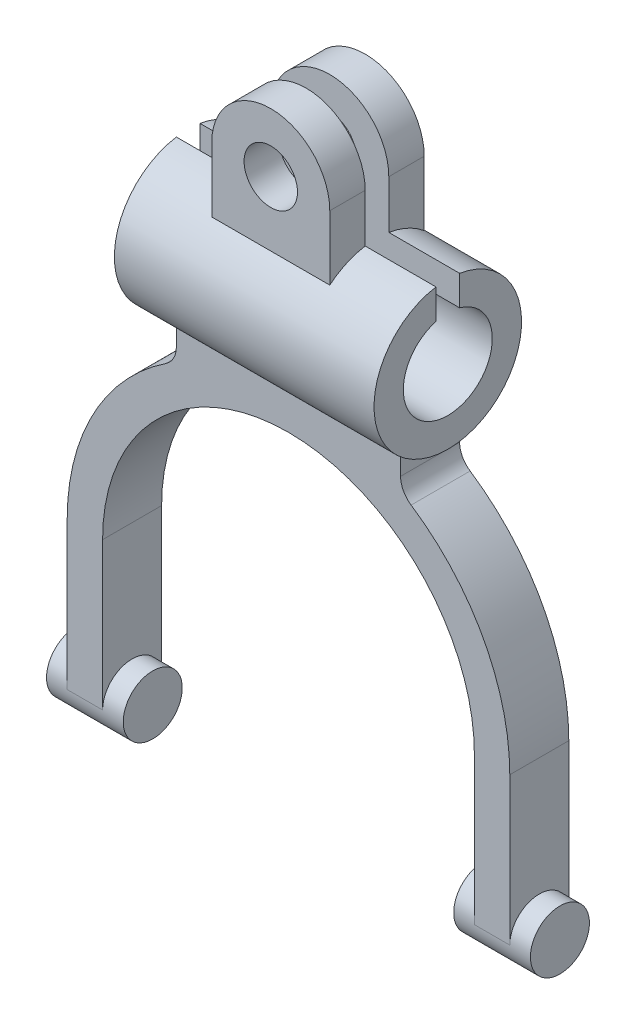
ISO-10303-21;
HEADER;
FILE_DESCRIPTION(('STEP AP214'),'2;1');
FILE_NAME('part.step','',(''),(''),'','','');
FILE_SCHEMA(('AUTOMOTIVE_DESIGN { 1 0 10303 214 1 1 1 1 }'));
ENDSEC;
DATA;
#1=APPLICATION_CONTEXT('core data for automotive mechanical design processes');
#2=APPLICATION_PROTOCOL_DEFINITION('international standard','automotive_design',2000,#1);
#3=PRODUCT_CONTEXT('',#1,'mechanical');
#4=PRODUCT('Part','Part','',(#3));
#5=PRODUCT_RELATED_PRODUCT_CATEGORY('part','',(#4));
#6=PRODUCT_DEFINITION_FORMATION('','',#4);
#7=PRODUCT_DEFINITION_CONTEXT('part definition',#1,'design');
#8=PRODUCT_DEFINITION('design','',#6,#7);
#9=PRODUCT_DEFINITION_SHAPE('','',#8);
#10=(LENGTH_UNIT() NAMED_UNIT(*) SI_UNIT(.MILLI.,.METRE.));
#11=(NAMED_UNIT(*) PLANE_ANGLE_UNIT() SI_UNIT($,.RADIAN.));
#12=(NAMED_UNIT(*) SI_UNIT($,.STERADIAN.) SOLID_ANGLE_UNIT());
#13=UNCERTAINTY_MEASURE_WITH_UNIT(LENGTH_MEASURE(1.E-05),#10,'distance_accuracy_value','');
#14=(GEOMETRIC_REPRESENTATION_CONTEXT(3) GLOBAL_UNCERTAINTY_ASSIGNED_CONTEXT((#13)) GLOBAL_UNIT_ASSIGNED_CONTEXT((#10,
#11,#12)) REPRESENTATION_CONTEXT('',''));
#15=CARTESIAN_POINT('',(0.,0.,0.));
#16=DIRECTION('',(0.,0.,1.));
#17=DIRECTION('',(1.,0.,0.));
#18=AXIS2_PLACEMENT_3D('',#15,#16,#17);
#19=CARTESIAN_POINT('',(22.,0.,5.));
#20=DIRECTION('',(-1.,0.,0.));
#21=DIRECTION('',(0.,0.,1.));
#22=AXIS2_PLACEMENT_3D('',#19,#20,#21);
#23=CYLINDRICAL_SURFACE('',#22,12.5);
#24=DIRECTION('',(-1.,0.,0.));
#25=VECTOR('',#24,1.);
#26=CARTESIAN_POINT('',(22.,-11.4564392373896,10.));
#27=LINE('',#26,#25);
#28=CARTESIAN_POINT('',(19.,-11.4564392373896,10.));
#29=VERTEX_POINT('',#28);
#30=CARTESIAN_POINT('',(-19.,-11.4564392373896,10.));
#31=VERTEX_POINT('',#30);
#32=EDGE_CURVE('E411',#29,#31,#27,.T.);
#33=ORIENTED_EDGE('',*,*,#32,.F.);
#34=CARTESIAN_POINT('',(19.,0.,5.));
#35=DIRECTION('',(1.,0.,0.));
#36=DIRECTION('',(0.,0.,-1.));
#37=AXIS2_PLACEMENT_3D('',#34,#35,#36);
#38=CIRCLE('',#37,12.5);
#39=CARTESIAN_POINT('',(19.,-11.4564392373896,0.));
#40=VERTEX_POINT('',#39);
#41=EDGE_CURVE('E413',#40,#29,#38,.F.);
#42=ORIENTED_EDGE('',*,*,#41,.F.);
#43=DIRECTION('',(-1.,0.,0.));
#44=VECTOR('',#43,1.);
#45=CARTESIAN_POINT('',(22.,-11.4564392373896,0.));
#46=LINE('',#45,#44);
#47=CARTESIAN_POINT('',(-19.,-11.4564392373896,0.));
#48=VERTEX_POINT('',#47);
#49=EDGE_CURVE('E307',#40,#48,#46,.T.);
#50=ORIENTED_EDGE('',*,*,#49,.T.);
#51=CARTESIAN_POINT('',(-19.,0.,5.));
#52=DIRECTION('',(1.,0.,0.));
#53=DIRECTION('',(0.,0.,-1.));
#54=AXIS2_PLACEMENT_3D('',#51,#52,#53);
#55=CIRCLE('',#54,12.5);
#56=EDGE_CURVE('E410',#48,#31,#55,.F.);
#57=ORIENTED_EDGE('',*,*,#56,.T.);
#58=EDGE_LOOP('',(#33,#42,#50,#57));
#59=FACE_BOUND('',#58,.T.);
#60=DIRECTION('',(-1.,0.,0.));
#61=VECTOR('',#60,1.);
#62=CARTESIAN_POINT('',(22.,9.60468635614927,-3.));
#63=LINE('',#62,#61);
#64=CARTESIAN_POINT('',(10.,9.60468635614927,-3.));
#65=VERTEX_POINT('',#64);
#66=CARTESIAN_POINT('',(-10.,9.60468635614927,-3.));
#67=VERTEX_POINT('',#66);
#68=EDGE_CURVE('E255',#65,#67,#63,.T.);
#69=ORIENTED_EDGE('',*,*,#68,.F.);
#70=CARTESIAN_POINT('',(10.,0.,5.));
#71=DIRECTION('',(1.,0.,0.));
#72=DIRECTION('',(0.,0.,-1.));
#73=AXIS2_PLACEMENT_3D('',#70,#71,#72);
#74=CIRCLE('',#73,12.5);
#75=CARTESIAN_POINT('',(10.,12.3389626792531,3.));
#76=VERTEX_POINT('',#75);
#77=EDGE_CURVE('E336',#65,#76,#74,.T.);
#78=ORIENTED_EDGE('',*,*,#77,.T.);
#79=DIRECTION('',(-1.,0.,0.));
#80=VECTOR('',#79,1.);
#81=CARTESIAN_POINT('',(22.,12.3389626792531,3.));
#82=LINE('',#81,#80);
#83=CARTESIAN_POINT('',(22.,12.3389626792531,3.));
#84=VERTEX_POINT('',#83);
#85=EDGE_CURVE('E403',#84,#76,#82,.T.);
#86=ORIENTED_EDGE('',*,*,#85,.F.);
#87=CARTESIAN_POINT('',(22.,0.,5.));
#88=DIRECTION('',(1.,0.,0.));
#89=DIRECTION('',(0.,0.,-1.));
#90=AXIS2_PLACEMENT_3D('',#87,#88,#89);
#91=CIRCLE('',#90,12.5);
#92=CARTESIAN_POINT('',(22.,12.3389626792531,7.));
#93=VERTEX_POINT('',#92);
#94=EDGE_CURVE('E378',#93,#84,#91,.T.);
#95=ORIENTED_EDGE('',*,*,#94,.F.);
#96=DIRECTION('',(-1.,0.,0.));
#97=VECTOR('',#96,1.);
#98=CARTESIAN_POINT('',(22.,12.3389626792531,7.));
#99=LINE('',#98,#97);
#100=CARTESIAN_POINT('',(10.,12.3389626792531,7.));
#101=VERTEX_POINT('',#100);
#102=EDGE_CURVE('E398',#93,#101,#99,.T.);
#103=ORIENTED_EDGE('',*,*,#102,.T.);
#104=CARTESIAN_POINT('',(10.,0.,5.));
#105=DIRECTION('',(-1.,0.,0.));
#106=DIRECTION('',(0.,0.,1.));
#107=AXIS2_PLACEMENT_3D('',#104,#105,#106);
#108=CIRCLE('',#107,12.5);
#109=CARTESIAN_POINT('',(10.,9.60468635614927,13.));
#110=VERTEX_POINT('',#109);
#111=EDGE_CURVE('E374',#110,#101,#108,.T.);
#112=ORIENTED_EDGE('',*,*,#111,.F.);
#113=DIRECTION('',(-1.,0.,0.));
#114=VECTOR('',#113,1.);
#115=CARTESIAN_POINT('',(22.,9.60468635614927,13.));
#116=LINE('',#115,#114);
#117=CARTESIAN_POINT('',(-10.,9.60468635614927,13.));
#118=VERTEX_POINT('',#117);
#119=EDGE_CURVE('E315',#118,#110,#116,.F.);
#120=ORIENTED_EDGE('',*,*,#119,.F.);
#121=CARTESIAN_POINT('',(-10.,0.,5.));
#122=DIRECTION('',(1.,0.,0.));
#123=DIRECTION('',(0.,1.,0.));
#124=AXIS2_PLACEMENT_3D('',#121,#122,#123);
#125=CIRCLE('',#124,12.5);
#126=CARTESIAN_POINT('',(-10.,12.3389626792531,7.));
#127=VERTEX_POINT('',#126);
#128=EDGE_CURVE('E375',#127,#118,#125,.T.);
#129=ORIENTED_EDGE('',*,*,#128,.F.);
#130=CARTESIAN_POINT('',(-22.,12.3389626792531,7.));
#131=VERTEX_POINT('',#130);
#132=EDGE_CURVE('E388',#127,#131,#99,.T.);
#133=ORIENTED_EDGE('',*,*,#132,.T.);
#134=CARTESIAN_POINT('',(-22.,0.,5.));
#135=DIRECTION('',(1.,0.,0.));
#136=DIRECTION('',(0.,0.,-1.));
#137=AXIS2_PLACEMENT_3D('',#134,#135,#136);
#138=CIRCLE('',#137,12.5);
#139=CARTESIAN_POINT('',(-22.,12.3389626792531,3.));
#140=VERTEX_POINT('',#139);
#141=EDGE_CURVE('E377',#131,#140,#138,.T.);
#142=ORIENTED_EDGE('',*,*,#141,.T.);
#143=CARTESIAN_POINT('',(-10.,12.3389626792531,3.));
#144=VERTEX_POINT('',#143);
#145=EDGE_CURVE('E340',#144,#140,#82,.T.);
#146=ORIENTED_EDGE('',*,*,#145,.F.);
#147=CARTESIAN_POINT('',(-10.,0.,5.));
#148=DIRECTION('',(-1.,0.,0.));
#149=DIRECTION('',(0.,0.,1.));
#150=AXIS2_PLACEMENT_3D('',#147,#148,#149);
#151=CIRCLE('',#150,12.5);
#152=EDGE_CURVE('E334',#144,#67,#151,.T.);
#153=ORIENTED_EDGE('',*,*,#152,.T.);
#154=EDGE_LOOP('',(#69,#78,#86,#95,#103,#112,#120,#129,#133,#142,#146,#153));
#155=FACE_BOUND('',#154,.T.);
#156=ADVANCED_FACE('F50',(#59,#155),#23,.T.);
#157=CARTESIAN_POINT('',(22.,0.,5.));
#158=DIRECTION('',(-1.,0.,0.));
#159=DIRECTION('',(0.,0.,1.));
#160=AXIS2_PLACEMENT_3D('',#157,#158,#159);
#161=CYLINDRICAL_SURFACE('',#160,7.54);
#162=CARTESIAN_POINT('',(-22.,0.,5.));
#163=DIRECTION('',(-1.,0.,0.));
#164=DIRECTION('',(0.,0.,-1.));
#165=AXIS2_PLACEMENT_3D('',#162,#163,#164);
#166=CIRCLE('',#165,7.54);
#167=CARTESIAN_POINT('',(-22.,7.26991059092201,3.));
#168=VERTEX_POINT('',#167);
#169=CARTESIAN_POINT('',(-22.,7.26991059092201,7.));
#170=VERTEX_POINT('',#169);
#171=EDGE_CURVE('E394',#168,#170,#166,.T.);
#172=ORIENTED_EDGE('',*,*,#171,.T.);
#173=DIRECTION('',(-1.,0.,0.));
#174=VECTOR('',#173,1.);
#175=CARTESIAN_POINT('',(22.,7.26991059092201,7.));
#176=LINE('',#175,#174);
#177=CARTESIAN_POINT('',(22.,7.26991059092201,7.));
#178=VERTEX_POINT('',#177);
#179=EDGE_CURVE('E402',#178,#170,#176,.T.);
#180=ORIENTED_EDGE('',*,*,#179,.F.);
#181=CARTESIAN_POINT('',(22.,0.,5.));
#182=DIRECTION('',(-1.,0.,0.));
#183=DIRECTION('',(0.,0.,-1.));
#184=AXIS2_PLACEMENT_3D('',#181,#182,#183);
#185=CIRCLE('',#184,7.54);
#186=CARTESIAN_POINT('',(22.,7.26991059092201,3.));
#187=VERTEX_POINT('',#186);
#188=EDGE_CURVE('E383',#187,#178,#185,.T.);
#189=ORIENTED_EDGE('',*,*,#188,.F.);
#190=DIRECTION('',(-1.,0.,0.));
#191=VECTOR('',#190,1.);
#192=CARTESIAN_POINT('',(22.,7.26991059092201,3.));
#193=LINE('',#192,#191);
#194=EDGE_CURVE('E401',#187,#168,#193,.T.);
#195=ORIENTED_EDGE('',*,*,#194,.T.);
#196=EDGE_LOOP('',(#172,#180,#189,#195));
#197=FACE_BOUND('',#196,.T.);
#198=ADVANCED_FACE('F505',(#197),#161,.F.);
#199=CARTESIAN_POINT('',(19.,0.,10.));
#200=DIRECTION('',(1.,0.,0.));
#201=DIRECTION('',(0.,0.,-1.));
#202=AXIS2_PLACEMENT_3D('',#199,#200,#201);
#203=PLANE('',#202);
#204=DIRECTION('',(0.,-1.,0.));
#205=VECTOR('',#204,1.);
#206=CARTESIAN_POINT('',(19.,0.,10.));
#207=LINE('',#206,#205);
#208=CARTESIAN_POINT('',(19.,-15.4537591050623,10.));
#209=VERTEX_POINT('',#208);
#210=EDGE_CURVE('E416',#29,#209,#207,.T.);
#211=ORIENTED_EDGE('',*,*,#210,.T.);
#212=DIRECTION('',(0.,0.,1.));
#213=VECTOR('',#212,1.);
#214=CARTESIAN_POINT('',(19.,-15.4537591050623,0.));
#215=LINE('',#214,#213);
#216=CARTESIAN_POINT('',(19.,-15.4537591050623,0.));
#217=VERTEX_POINT('',#216);
#218=EDGE_CURVE('E244',#209,#217,#215,.F.);
#219=ORIENTED_EDGE('',*,*,#218,.T.);
#220=DIRECTION('',(0.,-1.,0.));
#221=VECTOR('',#220,1.);
#222=CARTESIAN_POINT('',(19.,0.,0.));
#223=LINE('',#222,#221);
#224=EDGE_CURVE('E277',#40,#217,#223,.T.);
#225=ORIENTED_EDGE('',*,*,#224,.F.);
#226=ORIENTED_EDGE('',*,*,#41,.T.);
#227=EDGE_LOOP('',(#211,#219,#225,#226));
#228=FACE_BOUND('',#227,.T.);
#229=ADVANCED_FACE('F440',(#228),#203,.T.);
#230=CARTESIAN_POINT('',(-19.,0.,10.));
#231=DIRECTION('',(1.,0.,0.));
#232=DIRECTION('',(0.,0.,-1.));
#233=AXIS2_PLACEMENT_3D('',#230,#231,#232);
#234=PLANE('',#233);
#235=DIRECTION('',(0.,-1.,0.));
#236=VECTOR('',#235,1.);
#237=CARTESIAN_POINT('',(-19.,0.,0.));
#238=LINE('',#237,#236);
#239=CARTESIAN_POINT('',(-19.,-15.4593398311055,0.));
#240=VERTEX_POINT('',#239);
#241=EDGE_CURVE('E276',#48,#240,#238,.T.);
#242=ORIENTED_EDGE('',*,*,#241,.T.);
#243=DIRECTION('',(0.,0.,-1.));
#244=VECTOR('',#243,1.);
#245=CARTESIAN_POINT('',(-19.,-15.4593398311055,10.));
#246=LINE('',#245,#244);
#247=CARTESIAN_POINT('',(-19.,-15.4593398311055,10.));
#248=VERTEX_POINT('',#247);
#249=EDGE_CURVE('E61',#240,#248,#246,.F.);
#250=ORIENTED_EDGE('',*,*,#249,.T.);
#251=DIRECTION('',(0.,-1.,0.));
#252=VECTOR('',#251,1.);
#253=CARTESIAN_POINT('',(-19.,0.,10.));
#254=LINE('',#253,#252);
#255=EDGE_CURVE('E417',#31,#248,#254,.T.);
#256=ORIENTED_EDGE('',*,*,#255,.F.);
#257=ORIENTED_EDGE('',*,*,#56,.F.);
#258=EDGE_LOOP('',(#242,#250,#256,#257));
#259=FACE_BOUND('',#258,.T.);
#260=ADVANCED_FACE('F445',(#259),#234,.F.);
#261=CARTESIAN_POINT('',(0.,0.,10.));
#262=DIRECTION('',(0.,0.,1.));
#263=DIRECTION('',(1.,0.,0.));
#264=AXIS2_PLACEMENT_3D('',#261,#262,#263);
#265=PLANE('',#264);
#266=ORIENTED_EDGE('',*,*,#210,.F.);
#267=ORIENTED_EDGE('',*,*,#32,.T.);
#268=ORIENTED_EDGE('',*,*,#255,.T.);
#269=CARTESIAN_POINT('',(-23.,-15.4593398311055,10.));
#270=DIRECTION('',(0.,0.,1.));
#271=DIRECTION('',(1.,0.,0.));
#272=AXIS2_PLACEMENT_3D('',#269,#270,#271);
#273=CIRCLE('',#272,4.);
#274=CARTESIAN_POINT('',(-20.7827285960524,-18.7885600883483,10.));
#275=VERTEX_POINT('',#274);
#276=EDGE_CURVE('E11',#248,#275,#273,.F.);
#277=ORIENTED_EDGE('',*,*,#276,.T.);
#278=CARTESIAN_POINT('',(0.00419081595661591,-50.,10.));
#279=DIRECTION('',(0.,0.,1.));
#280=DIRECTION('',(1.,0.,0.));
#281=AXIS2_PLACEMENT_3D('',#278,#279,#280);
#282=CIRCLE('',#281,37.5);
#283=CARTESIAN_POINT('',(-37.4958091840434,-50.,10.));
#284=VERTEX_POINT('',#283);
#285=EDGE_CURVE('E272',#284,#275,#282,.F.);
#286=ORIENTED_EDGE('',*,*,#285,.F.);
#287=DIRECTION('',(0.,1.,0.));
#288=VECTOR('',#287,1.);
#289=CARTESIAN_POINT('',(-37.4958091840434,0.,10.));
#290=LINE('',#289,#288);
#291=CARTESIAN_POINT('',(-37.4958091840434,-75.,10.));
#292=VERTEX_POINT('',#291);
#293=EDGE_CURVE('E240',#292,#284,#290,.T.);
#294=ORIENTED_EDGE('',*,*,#293,.F.);
#295=DIRECTION('',(1.,0.,0.));
#296=VECTOR('',#295,1.);
#297=CARTESIAN_POINT('',(0.,-75.,10.));
#298=LINE('',#297,#296);
#299=CARTESIAN_POINT('',(-31.4958091840434,-75.,10.));
#300=VERTEX_POINT('',#299);
#301=EDGE_CURVE('E230',#292,#300,#298,.T.);
#302=ORIENTED_EDGE('',*,*,#301,.T.);
#303=DIRECTION('',(0.,1.,0.));
#304=VECTOR('',#303,1.);
#305=CARTESIAN_POINT('',(-31.4958091840434,0.,10.));
#306=LINE('',#305,#304);
#307=CARTESIAN_POINT('',(-31.4958091840434,-50.,10.));
#308=VERTEX_POINT('',#307);
#309=EDGE_CURVE('E216',#300,#308,#306,.T.);
#310=ORIENTED_EDGE('',*,*,#309,.T.);
#311=CARTESIAN_POINT('',(0.00419081595661591,-50.,10.));
#312=DIRECTION('',(0.,0.,1.));
#313=DIRECTION('',(1.,0.,0.));
#314=AXIS2_PLACEMENT_3D('',#311,#312,#313);
#315=CIRCLE('',#314,31.5);
#316=CARTESIAN_POINT('',(31.5041908159566,-50.,10.));
#317=VERTEX_POINT('',#316);
#318=EDGE_CURVE('E226',#308,#317,#315,.F.);
#319=ORIENTED_EDGE('',*,*,#318,.T.);
#320=DIRECTION('',(0.,-1.,0.));
#321=VECTOR('',#320,1.);
#322=CARTESIAN_POINT('',(31.5041908159566,0.,10.));
#323=LINE('',#322,#321);
#324=CARTESIAN_POINT('',(31.5041908159566,-75.,10.));
#325=VERTEX_POINT('',#324);
#326=EDGE_CURVE('E424',#317,#325,#323,.T.);
#327=ORIENTED_EDGE('',*,*,#326,.T.);
#328=DIRECTION('',(-1.,0.,0.));
#329=VECTOR('',#328,1.);
#330=CARTESIAN_POINT('',(0.,-75.,10.));
#331=LINE('',#330,#329);
#332=CARTESIAN_POINT('',(37.5041908159566,-75.,10.));
#333=VERTEX_POINT('',#332);
#334=EDGE_CURVE('E426',#333,#325,#331,.T.);
#335=ORIENTED_EDGE('',*,*,#334,.F.);
#336=DIRECTION('',(0.,-1.,0.));
#337=VECTOR('',#336,1.);
#338=CARTESIAN_POINT('',(37.5041908159566,0.,10.));
#339=LINE('',#338,#337);
#340=CARTESIAN_POINT('',(37.5041908159566,-50.,10.));
#341=VERTEX_POINT('',#340);
#342=EDGE_CURVE('E303',#341,#333,#339,.T.);
#343=ORIENTED_EDGE('',*,*,#342,.F.);
#344=CARTESIAN_POINT('',(0.00419081595661591,-50.,10.));
#345=DIRECTION('',(0.,0.,1.));
#346=DIRECTION('',(1.,0.,0.));
#347=AXIS2_PLACEMENT_3D('',#344,#345,#346);
#348=CIRCLE('',#347,37.5);
#349=CARTESIAN_POINT('',(20.7835364641886,-18.7835172636105,10.));
#350=VERTEX_POINT('',#349);
#351=EDGE_CURVE('E296',#350,#341,#348,.F.);
#352=ORIENTED_EDGE('',*,*,#351,.F.);
#353=CARTESIAN_POINT('',(23.,-15.4537591050623,10.));
#354=DIRECTION('',(0.,0.,1.));
#355=DIRECTION('',(1.,0.,0.));
#356=AXIS2_PLACEMENT_3D('',#353,#354,#355);
#357=CIRCLE('',#356,4.);
#358=EDGE_CURVE('E258',#350,#209,#357,.F.);
#359=ORIENTED_EDGE('',*,*,#358,.T.);
#360=EDGE_LOOP('',(#266,#267,#268,#277,#286,#294,#302,#310,#319,#327,#335,#343,#352,#359));
#361=FACE_BOUND('',#360,.T.);
#362=ADVANCED_FACE('F234',(#361),#265,.T.);
#363=CARTESIAN_POINT('',(0.,0.,0.));
#364=DIRECTION('',(0.,0.,1.));
#365=DIRECTION('',(1.,0.,0.));
#366=AXIS2_PLACEMENT_3D('',#363,#364,#365);
#367=PLANE('',#366);
#368=ORIENTED_EDGE('',*,*,#49,.F.);
#369=ORIENTED_EDGE('',*,*,#224,.T.);
#370=CARTESIAN_POINT('',(23.,-15.4537591050623,0.));
#371=DIRECTION('',(0.,0.,1.));
#372=DIRECTION('',(1.,0.,0.));
#373=AXIS2_PLACEMENT_3D('',#370,#371,#372);
#374=CIRCLE('',#373,4.);
#375=CARTESIAN_POINT('',(20.7835364641886,-18.7835172636105,0.));
#376=VERTEX_POINT('',#375);
#377=EDGE_CURVE('E256',#217,#376,#374,.T.);
#378=ORIENTED_EDGE('',*,*,#377,.T.);
#379=CARTESIAN_POINT('',(0.00419081595661591,-50.,0.));
#380=DIRECTION('',(0.,0.,1.));
#381=DIRECTION('',(1.,0.,0.));
#382=AXIS2_PLACEMENT_3D('',#379,#380,#381);
#383=CIRCLE('',#382,37.5);
#384=CARTESIAN_POINT('',(37.5041908159566,-50.,0.));
#385=VERTEX_POINT('',#384);
#386=EDGE_CURVE('E412',#376,#385,#383,.F.);
#387=ORIENTED_EDGE('',*,*,#386,.T.);
#388=DIRECTION('',(0.,-1.,0.));
#389=VECTOR('',#388,1.);
#390=CARTESIAN_POINT('',(37.5041908159566,0.,0.));
#391=LINE('',#390,#389);
#392=CARTESIAN_POINT('',(37.5041908159566,-75.,0.));
#393=VERTEX_POINT('',#392);
#394=EDGE_CURVE('E294',#385,#393,#391,.T.);
#395=ORIENTED_EDGE('',*,*,#394,.T.);
#396=DIRECTION('',(-1.,0.,0.));
#397=VECTOR('',#396,1.);
#398=CARTESIAN_POINT('',(0.,-75.,0.));
#399=LINE('',#398,#397);
#400=CARTESIAN_POINT('',(31.5041908159566,-75.,0.));
#401=VERTEX_POINT('',#400);
#402=EDGE_CURVE('E292',#393,#401,#399,.T.);
#403=ORIENTED_EDGE('',*,*,#402,.T.);
#404=DIRECTION('',(0.,-1.,0.));
#405=VECTOR('',#404,1.);
#406=CARTESIAN_POINT('',(31.5041908159566,0.,0.));
#407=LINE('',#406,#405);
#408=CARTESIAN_POINT('',(31.5041908159566,-50.,0.));
#409=VERTEX_POINT('',#408);
#410=EDGE_CURVE('E288',#409,#401,#407,.T.);
#411=ORIENTED_EDGE('',*,*,#410,.F.);
#412=CARTESIAN_POINT('',(0.00419081595661591,-50.,0.));
#413=DIRECTION('',(0.,0.,1.));
#414=DIRECTION('',(1.,0.,0.));
#415=AXIS2_PLACEMENT_3D('',#412,#413,#414);
#416=CIRCLE('',#415,31.5);
#417=CARTESIAN_POINT('',(-31.4958091840434,-50.,0.));
#418=VERTEX_POINT('',#417);
#419=EDGE_CURVE('E286',#418,#409,#416,.F.);
#420=ORIENTED_EDGE('',*,*,#419,.F.);
#421=DIRECTION('',(0.,1.,0.));
#422=VECTOR('',#421,1.);
#423=CARTESIAN_POINT('',(-31.4958091840434,0.,0.));
#424=LINE('',#423,#422);
#425=CARTESIAN_POINT('',(-31.4958091840434,-75.,0.));
#426=VERTEX_POINT('',#425);
#427=EDGE_CURVE('E282',#426,#418,#424,.T.);
#428=ORIENTED_EDGE('',*,*,#427,.F.);
#429=DIRECTION('',(1.,0.,0.));
#430=VECTOR('',#429,1.);
#431=CARTESIAN_POINT('',(0.,-75.,0.));
#432=LINE('',#431,#430);
#433=CARTESIAN_POINT('',(-37.4958091840434,-75.,0.));
#434=VERTEX_POINT('',#433);
#435=EDGE_CURVE('E242',#434,#426,#432,.T.);
#436=ORIENTED_EDGE('',*,*,#435,.F.);
#437=DIRECTION('',(0.,1.,0.));
#438=VECTOR('',#437,1.);
#439=CARTESIAN_POINT('',(-37.4958091840434,0.,0.));
#440=LINE('',#439,#438);
#441=CARTESIAN_POINT('',(-37.4958091840434,-50.,0.));
#442=VERTEX_POINT('',#441);
#443=EDGE_CURVE('E279',#434,#442,#440,.T.);
#444=ORIENTED_EDGE('',*,*,#443,.T.);
#445=CARTESIAN_POINT('',(0.00419081595661591,-50.,0.));
#446=DIRECTION('',(0.,0.,1.));
#447=DIRECTION('',(1.,0.,0.));
#448=AXIS2_PLACEMENT_3D('',#445,#446,#447);
#449=CIRCLE('',#448,37.5);
#450=CARTESIAN_POINT('',(-20.7827285960524,-18.7885600883483,0.));
#451=VERTEX_POINT('',#450);
#452=EDGE_CURVE('E268',#442,#451,#449,.F.);
#453=ORIENTED_EDGE('',*,*,#452,.T.);
#454=CARTESIAN_POINT('',(-23.,-15.4593398311055,0.));
#455=DIRECTION('',(0.,0.,1.));
#456=DIRECTION('',(1.,0.,0.));
#457=AXIS2_PLACEMENT_3D('',#454,#455,#456);
#458=CIRCLE('',#457,4.);
#459=EDGE_CURVE('E54',#451,#240,#458,.T.);
#460=ORIENTED_EDGE('',*,*,#459,.T.);
#461=ORIENTED_EDGE('',*,*,#241,.F.);
#462=EDGE_LOOP('',(#368,#369,#378,#387,#395,#403,#411,#420,#428,#436,#444,#453,#460,#461));
#463=FACE_BOUND('',#462,.T.);
#464=ADVANCED_FACE('F274',(#463),#367,.F.);
#465=CARTESIAN_POINT('',(0.00419081595661591,-50.,10.));
#466=DIRECTION('',(0.,0.,-1.));
#467=DIRECTION('',(-1.,0.,0.));
#468=AXIS2_PLACEMENT_3D('',#465,#466,#467);
#469=CYLINDRICAL_SURFACE('',#468,37.5);
#470=ORIENTED_EDGE('',*,*,#386,.F.);
#471=DIRECTION('',(0.,0.,-1.));
#472=VECTOR('',#471,1.);
#473=CARTESIAN_POINT('',(20.7835364641886,-18.7835172636105,10.));
#474=LINE('',#473,#472);
#475=EDGE_CURVE('E248',#376,#350,#474,.F.);
#476=ORIENTED_EDGE('',*,*,#475,.T.);
#477=ORIENTED_EDGE('',*,*,#351,.T.);
#478=DIRECTION('',(0.,0.,-1.));
#479=VECTOR('',#478,1.);
#480=CARTESIAN_POINT('',(37.5041908159566,-50.,10.));
#481=LINE('',#480,#479);
#482=EDGE_CURVE('E299',#341,#385,#481,.T.);
#483=ORIENTED_EDGE('',*,*,#482,.T.);
#484=EDGE_LOOP('',(#470,#476,#477,#483));
#485=FACE_BOUND('',#484,.T.);
#486=ADVANCED_FACE('F542',(#485),#469,.T.);
#487=CARTESIAN_POINT('',(0.00419081595661591,-50.,10.));
#488=DIRECTION('',(0.,0.,-1.));
#489=DIRECTION('',(-1.,0.,0.));
#490=AXIS2_PLACEMENT_3D('',#487,#488,#489);
#491=CYLINDRICAL_SURFACE('',#490,37.5);
#492=ORIENTED_EDGE('',*,*,#285,.T.);
#493=DIRECTION('',(0.,0.,-1.));
#494=VECTOR('',#493,1.);
#495=CARTESIAN_POINT('',(-20.7827285960524,-18.7885600883483,10.));
#496=LINE('',#495,#494);
#497=EDGE_CURVE('E263',#275,#451,#496,.T.);
#498=ORIENTED_EDGE('',*,*,#497,.T.);
#499=ORIENTED_EDGE('',*,*,#452,.F.);
#500=DIRECTION('',(0.,0.,-1.));
#501=VECTOR('',#500,1.);
#502=CARTESIAN_POINT('',(-37.4958091840434,-50.,10.));
#503=LINE('',#502,#501);
#504=EDGE_CURVE('E310',#284,#442,#503,.T.);
#505=ORIENTED_EDGE('',*,*,#504,.F.);
#506=EDGE_LOOP('',(#492,#498,#499,#505));
#507=FACE_BOUND('',#506,.T.);
#508=ADVANCED_FACE('F270',(#507),#491,.T.);
#509=CARTESIAN_POINT('',(-37.4958091840434,0.,10.));
#510=DIRECTION('',(-1.,0.,0.));
#511=DIRECTION('',(0.,0.,1.));
#512=AXIS2_PLACEMENT_3D('',#509,#510,#511);
#513=PLANE('',#512);
#514=ORIENTED_EDGE('',*,*,#443,.F.);
#515=CARTESIAN_POINT('',(-37.4958091840434,-75.,5.));
#516=DIRECTION('',(-1.,0.,0.));
#517=DIRECTION('',(0.,0.,1.));
#518=AXIS2_PLACEMENT_3D('',#515,#516,#517);
#519=CIRCLE('',#518,5.);
#520=EDGE_CURVE('E444',#434,#292,#519,.F.);
#521=ORIENTED_EDGE('',*,*,#520,.T.);
#522=ORIENTED_EDGE('',*,*,#293,.T.);
#523=ORIENTED_EDGE('',*,*,#504,.T.);
#524=EDGE_LOOP('',(#514,#521,#522,#523));
#525=FACE_BOUND('',#524,.T.);
#526=ADVANCED_FACE('F443',(#525),#513,.T.);
#527=CARTESIAN_POINT('',(-31.4958091840434,0.,10.));
#528=DIRECTION('',(-1.,0.,0.));
#529=DIRECTION('',(0.,0.,1.));
#530=AXIS2_PLACEMENT_3D('',#527,#528,#529);
#531=PLANE('',#530);
#532=CARTESIAN_POINT('',(-31.4958091840434,-75.,5.));
#533=DIRECTION('',(-1.,0.,0.));
#534=DIRECTION('',(0.,0.,1.));
#535=AXIS2_PLACEMENT_3D('',#532,#533,#534);
#536=CIRCLE('',#535,5.);
#537=EDGE_CURVE('E221',#426,#300,#536,.F.);
#538=ORIENTED_EDGE('',*,*,#537,.F.);
#539=ORIENTED_EDGE('',*,*,#427,.T.);
#540=DIRECTION('',(0.,0.,-1.));
#541=VECTOR('',#540,1.);
#542=CARTESIAN_POINT('',(-31.4958091840434,-50.,10.));
#543=LINE('',#542,#541);
#544=EDGE_CURVE('E222',#308,#418,#543,.T.);
#545=ORIENTED_EDGE('',*,*,#544,.F.);
#546=ORIENTED_EDGE('',*,*,#309,.F.);
#547=EDGE_LOOP('',(#538,#539,#545,#546));
#548=FACE_BOUND('',#547,.T.);
#549=ADVANCED_FACE('F217',(#548),#531,.F.);
#550=CARTESIAN_POINT('',(0.00419081595661591,-50.,10.));
#551=DIRECTION('',(0.,0.,-1.));
#552=DIRECTION('',(-1.,0.,0.));
#553=AXIS2_PLACEMENT_3D('',#550,#551,#552);
#554=CYLINDRICAL_SURFACE('',#553,31.5);
#555=ORIENTED_EDGE('',*,*,#419,.T.);
#556=DIRECTION('',(0.,0.,-1.));
#557=VECTOR('',#556,1.);
#558=CARTESIAN_POINT('',(31.5041908159566,-50.,10.));
#559=LINE('',#558,#557);
#560=EDGE_CURVE('E305',#317,#409,#559,.T.);
#561=ORIENTED_EDGE('',*,*,#560,.F.);
#562=ORIENTED_EDGE('',*,*,#318,.F.);
#563=ORIENTED_EDGE('',*,*,#544,.T.);
#564=EDGE_LOOP('',(#555,#561,#562,#563));
#565=FACE_BOUND('',#564,.T.);
#566=ADVANCED_FACE('F551',(#565),#554,.F.);
#567=CARTESIAN_POINT('',(31.5041908159566,0.,10.));
#568=DIRECTION('',(1.,0.,0.));
#569=DIRECTION('',(0.,0.,-1.));
#570=AXIS2_PLACEMENT_3D('',#567,#568,#569);
#571=PLANE('',#570);
#572=CARTESIAN_POINT('',(31.5041908159566,-75.,5.));
#573=DIRECTION('',(1.,0.,0.));
#574=DIRECTION('',(0.,0.,-1.));
#575=AXIS2_PLACEMENT_3D('',#572,#573,#574);
#576=CIRCLE('',#575,5.);
#577=EDGE_CURVE('E456',#325,#401,#576,.F.);
#578=ORIENTED_EDGE('',*,*,#577,.F.);
#579=ORIENTED_EDGE('',*,*,#326,.F.);
#580=ORIENTED_EDGE('',*,*,#560,.T.);
#581=ORIENTED_EDGE('',*,*,#410,.T.);
#582=EDGE_LOOP('',(#578,#579,#580,#581));
#583=FACE_BOUND('',#582,.T.);
#584=ADVANCED_FACE('F548',(#583),#571,.F.);
#585=CARTESIAN_POINT('',(37.5041908159566,0.,10.));
#586=DIRECTION('',(1.,0.,0.));
#587=DIRECTION('',(0.,0.,-1.));
#588=AXIS2_PLACEMENT_3D('',#585,#586,#587);
#589=PLANE('',#588);
#590=ORIENTED_EDGE('',*,*,#342,.T.);
#591=CARTESIAN_POINT('',(37.5041908159566,-75.,5.));
#592=DIRECTION('',(1.,0.,0.));
#593=DIRECTION('',(0.,0.,-1.));
#594=AXIS2_PLACEMENT_3D('',#591,#592,#593);
#595=CIRCLE('',#594,5.);
#596=EDGE_CURVE('E246',#333,#393,#595,.F.);
#597=ORIENTED_EDGE('',*,*,#596,.T.);
#598=ORIENTED_EDGE('',*,*,#394,.F.);
#599=ORIENTED_EDGE('',*,*,#482,.F.);
#600=EDGE_LOOP('',(#590,#597,#598,#599));
#601=FACE_BOUND('',#600,.T.);
#602=ADVANCED_FACE('F549',(#601),#589,.T.);
#603=CARTESIAN_POINT('',(22.,7.26991059092201,3.));
#604=DIRECTION('',(0.,0.,-1.));
#605=DIRECTION('',(-1.,0.,0.));
#606=AXIS2_PLACEMENT_3D('',#603,#604,#605);
#607=PLANE('',#606);
#608=DIRECTION('',(0.,-1.,0.));
#609=VECTOR('',#608,1.);
#610=CARTESIAN_POINT('',(-22.,7.26991059092201,3.));
#611=LINE('',#610,#609);
#612=EDGE_CURVE('E393',#140,#168,#611,.T.);
#613=ORIENTED_EDGE('',*,*,#612,.T.);
#614=ORIENTED_EDGE('',*,*,#194,.F.);
#615=DIRECTION('',(0.,-1.,0.));
#616=VECTOR('',#615,1.);
#617=CARTESIAN_POINT('',(22.,7.26991059092201,3.));
#618=LINE('',#617,#616);
#619=EDGE_CURVE('E385',#84,#187,#618,.T.);
#620=ORIENTED_EDGE('',*,*,#619,.F.);
#621=ORIENTED_EDGE('',*,*,#85,.T.);
#622=DIRECTION('',(0.,1.,0.));
#623=VECTOR('',#622,1.);
#624=CARTESIAN_POINT('',(10.,20.5161785694575,3.));
#625=LINE('',#624,#623);
#626=CARTESIAN_POINT('',(10.,20.5161785694575,3.));
#627=VERTEX_POINT('',#626);
#628=EDGE_CURVE('E466',#76,#627,#625,.T.);
#629=ORIENTED_EDGE('',*,*,#628,.T.);
#630=CARTESIAN_POINT('',(0.,20.5161785694575,3.));
#631=DIRECTION('',(0.,0.,1.));
#632=DIRECTION('',(1.,0.,0.));
#633=AXIS2_PLACEMENT_3D('',#630,#631,#632);
#634=CIRCLE('',#633,10.);
#635=CARTESIAN_POINT('',(-10.,20.5161785694575,3.));
#636=VERTEX_POINT('',#635);
#637=EDGE_CURVE('E462',#627,#636,#634,.T.);
#638=ORIENTED_EDGE('',*,*,#637,.T.);
#639=DIRECTION('',(0.,-1.,0.));
#640=VECTOR('',#639,1.);
#641=CARTESIAN_POINT('',(-10.,5.51617856945754,3.));
#642=LINE('',#641,#640);
#643=EDGE_CURVE('E475',#636,#144,#642,.T.);
#644=ORIENTED_EDGE('',*,*,#643,.T.);
#645=ORIENTED_EDGE('',*,*,#145,.T.);
#646=EDGE_LOOP('',(#613,#614,#620,#621,#629,#638,#644,#645));
#647=FACE_BOUND('',#646,.T.);
#648=CARTESIAN_POINT('',(0.,20.5161785694575,3.));
#649=DIRECTION('',(0.,0.,1.));
#650=DIRECTION('',(1.,0.,0.));
#651=AXIS2_PLACEMENT_3D('',#648,#649,#650);
#652=CIRCLE('',#651,4.525);
#653=CARTESIAN_POINT('',(4.525,20.5161785694575,3.));
#654=VERTEX_POINT('',#653);
#655=EDGE_CURVE('E464',#654,#654,#652,.T.);
#656=ORIENTED_EDGE('',*,*,#655,.F.);
#657=EDGE_LOOP('',(#656));
#658=FACE_BOUND('',#657,.T.);
#659=ADVANCED_FACE('F478',(#647,#658),#607,.F.);
#660=CARTESIAN_POINT('',(22.,7.26991059092201,7.));
#661=DIRECTION('',(0.,0.,1.));
#662=DIRECTION('',(1.,0.,0.));
#663=AXIS2_PLACEMENT_3D('',#660,#661,#662);
#664=PLANE('',#663);
#665=ORIENTED_EDGE('',*,*,#179,.T.);
#666=DIRECTION('',(0.,1.,0.));
#667=VECTOR('',#666,1.);
#668=CARTESIAN_POINT('',(-22.,7.26991059092201,7.));
#669=LINE('',#668,#667);
#670=EDGE_CURVE('E384',#170,#131,#669,.T.);
#671=ORIENTED_EDGE('',*,*,#670,.T.);
#672=ORIENTED_EDGE('',*,*,#132,.F.);
#673=DIRECTION('',(0.,-1.,0.));
#674=VECTOR('',#673,1.);
#675=CARTESIAN_POINT('',(-10.,5.51617856945754,7.));
#676=LINE('',#675,#674);
#677=CARTESIAN_POINT('',(-10.,20.5161785694575,7.));
#678=VERTEX_POINT('',#677);
#679=EDGE_CURVE('E358',#678,#127,#676,.T.);
#680=ORIENTED_EDGE('',*,*,#679,.F.);
#681=CARTESIAN_POINT('',(0.,20.5161785694575,7.));
#682=DIRECTION('',(0.,0.,1.));
#683=DIRECTION('',(-1.,0.,0.));
#684=AXIS2_PLACEMENT_3D('',#681,#682,#683);
#685=CIRCLE('',#684,10.);
#686=CARTESIAN_POINT('',(10.,20.5161785694575,7.));
#687=VERTEX_POINT('',#686);
#688=EDGE_CURVE('E361',#687,#678,#685,.T.);
#689=ORIENTED_EDGE('',*,*,#688,.F.);
#690=DIRECTION('',(0.,1.,0.));
#691=VECTOR('',#690,1.);
#692=CARTESIAN_POINT('',(10.,5.51617856945754,7.));
#693=LINE('',#692,#691);
#694=EDGE_CURVE('E347',#101,#687,#693,.T.);
#695=ORIENTED_EDGE('',*,*,#694,.F.);
#696=ORIENTED_EDGE('',*,*,#102,.F.);
#697=DIRECTION('',(0.,1.,0.));
#698=VECTOR('',#697,1.);
#699=CARTESIAN_POINT('',(22.,7.26991059092201,7.));
#700=LINE('',#699,#698);
#701=EDGE_CURVE('E386',#178,#93,#700,.T.);
#702=ORIENTED_EDGE('',*,*,#701,.F.);
#703=EDGE_LOOP('',(#665,#671,#672,#680,#689,#695,#696,#702));
#704=FACE_BOUND('',#703,.T.);
#705=CARTESIAN_POINT('',(0.,20.5161785694575,7.));
#706=DIRECTION('',(0.,0.,1.));
#707=DIRECTION('',(1.,0.,0.));
#708=AXIS2_PLACEMENT_3D('',#705,#706,#707);
#709=CIRCLE('',#708,4.525);
#710=CARTESIAN_POINT('',(4.525,20.5161785694575,7.));
#711=VERTEX_POINT('',#710);
#712=EDGE_CURVE('E344',#711,#711,#709,.T.);
#713=ORIENTED_EDGE('',*,*,#712,.T.);
#714=EDGE_LOOP('',(#713));
#715=FACE_BOUND('',#714,.T.);
#716=ADVANCED_FACE('F492',(#704,#715),#664,.F.);
#717=CARTESIAN_POINT('',(22.,0.,5.));
#718=DIRECTION('',(1.,0.,0.));
#719=DIRECTION('',(0.,0.,-1.));
#720=AXIS2_PLACEMENT_3D('',#717,#718,#719);
#721=PLANE('',#720);
#722=ORIENTED_EDGE('',*,*,#94,.T.);
#723=ORIENTED_EDGE('',*,*,#619,.T.);
#724=ORIENTED_EDGE('',*,*,#188,.T.);
#725=ORIENTED_EDGE('',*,*,#701,.T.);
#726=EDGE_LOOP('',(#722,#723,#724,#725));
#727=FACE_BOUND('',#726,.T.);
#728=ADVANCED_FACE('F504',(#727),#721,.T.);
#729=CARTESIAN_POINT('',(-22.,0.,5.));
#730=DIRECTION('',(1.,0.,0.));
#731=DIRECTION('',(0.,0.,-1.));
#732=AXIS2_PLACEMENT_3D('',#729,#730,#731);
#733=PLANE('',#732);
#734=ORIENTED_EDGE('',*,*,#141,.F.);
#735=ORIENTED_EDGE('',*,*,#670,.F.);
#736=ORIENTED_EDGE('',*,*,#171,.F.);
#737=ORIENTED_EDGE('',*,*,#612,.F.);
#738=EDGE_LOOP('',(#734,#735,#736,#737));
#739=FACE_BOUND('',#738,.T.);
#740=ADVANCED_FACE('F489',(#739),#733,.F.);
#741=CARTESIAN_POINT('',(0.,20.5161785694575,13.));
#742=DIRECTION('',(0.,0.,-1.));
#743=DIRECTION('',(-1.,0.,0.));
#744=AXIS2_PLACEMENT_3D('',#741,#742,#743);
#745=PLANE('',#744);
#746=CARTESIAN_POINT('',(0.,20.5161785694575,13.));
#747=DIRECTION('',(0.,0.,1.));
#748=DIRECTION('',(1.,0.,0.));
#749=AXIS2_PLACEMENT_3D('',#746,#747,#748);
#750=CIRCLE('',#749,4.525);
#751=CARTESIAN_POINT('',(4.525,20.5161785694575,13.));
#752=VERTEX_POINT('',#751);
#753=EDGE_CURVE('E350',#752,#752,#750,.T.);
#754=ORIENTED_EDGE('',*,*,#753,.F.);
#755=EDGE_LOOP('',(#754));
#756=FACE_BOUND('',#755,.T.);
#757=DIRECTION('',(0.,-1.,0.));
#758=VECTOR('',#757,1.);
#759=CARTESIAN_POINT('',(-10.,5.51617856945754,13.));
#760=LINE('',#759,#758);
#761=CARTESIAN_POINT('',(-10.,20.5161785694575,13.));
#762=VERTEX_POINT('',#761);
#763=EDGE_CURVE('E356',#762,#118,#760,.T.);
#764=ORIENTED_EDGE('',*,*,#763,.T.);
#765=ORIENTED_EDGE('',*,*,#119,.T.);
#766=DIRECTION('',(0.,1.,0.));
#767=VECTOR('',#766,1.);
#768=CARTESIAN_POINT('',(10.,5.51617856945754,13.));
#769=LINE('',#768,#767);
#770=CARTESIAN_POINT('',(10.,20.5161785694575,13.));
#771=VERTEX_POINT('',#770);
#772=EDGE_CURVE('E355',#110,#771,#769,.T.);
#773=ORIENTED_EDGE('',*,*,#772,.T.);
#774=CARTESIAN_POINT('',(0.,20.5161785694575,13.));
#775=DIRECTION('',(0.,0.,1.));
#776=DIRECTION('',(-1.,0.,0.));
#777=AXIS2_PLACEMENT_3D('',#774,#775,#776);
#778=CIRCLE('',#777,10.);
#779=EDGE_CURVE('E352',#771,#762,#778,.T.);
#780=ORIENTED_EDGE('',*,*,#779,.T.);
#781=EDGE_LOOP('',(#764,#765,#773,#780));
#782=FACE_BOUND('',#781,.T.);
#783=ADVANCED_FACE('F520',(#756,#782),#745,.F.);
#784=CARTESIAN_POINT('',(10.,5.51617856945754,13.));
#785=DIRECTION('',(-1.,0.,0.));
#786=DIRECTION('',(0.,0.,1.));
#787=AXIS2_PLACEMENT_3D('',#784,#785,#786);
#788=PLANE('',#787);
#789=ORIENTED_EDGE('',*,*,#772,.F.);
#790=ORIENTED_EDGE('',*,*,#111,.T.);
#791=ORIENTED_EDGE('',*,*,#694,.T.);
#792=DIRECTION('',(0.,0.,-1.));
#793=VECTOR('',#792,1.);
#794=CARTESIAN_POINT('',(10.,20.5161785694575,13.));
#795=LINE('',#794,#793);
#796=EDGE_CURVE('E367',#771,#687,#795,.T.);
#797=ORIENTED_EDGE('',*,*,#796,.F.);
#798=EDGE_LOOP('',(#789,#790,#791,#797));
#799=FACE_BOUND('',#798,.T.);
#800=ADVANCED_FACE('F508',(#799),#788,.F.);
#801=CARTESIAN_POINT('',(-10.,5.51617856945754,13.));
#802=DIRECTION('',(1.,0.,0.));
#803=DIRECTION('',(0.,1.,0.));
#804=AXIS2_PLACEMENT_3D('',#801,#802,#803);
#805=PLANE('',#804);
#806=ORIENTED_EDGE('',*,*,#679,.T.);
#807=ORIENTED_EDGE('',*,*,#128,.T.);
#808=ORIENTED_EDGE('',*,*,#763,.F.);
#809=DIRECTION('',(0.,0.,-1.));
#810=VECTOR('',#809,1.);
#811=CARTESIAN_POINT('',(-10.,20.5161785694575,13.));
#812=LINE('',#811,#810);
#813=EDGE_CURVE('E363',#762,#678,#812,.T.);
#814=ORIENTED_EDGE('',*,*,#813,.T.);
#815=EDGE_LOOP('',(#806,#807,#808,#814));
#816=FACE_BOUND('',#815,.T.);
#817=ADVANCED_FACE('F517',(#816),#805,.F.);
#818=CARTESIAN_POINT('',(0.,20.5161785694575,13.));
#819=DIRECTION('',(0.,0.,-1.));
#820=DIRECTION('',(-1.,0.,0.));
#821=AXIS2_PLACEMENT_3D('',#818,#819,#820);
#822=CYLINDRICAL_SURFACE('',#821,10.);
#823=ORIENTED_EDGE('',*,*,#688,.T.);
#824=ORIENTED_EDGE('',*,*,#813,.F.);
#825=ORIENTED_EDGE('',*,*,#779,.F.);
#826=ORIENTED_EDGE('',*,*,#796,.T.);
#827=EDGE_LOOP('',(#823,#824,#825,#826));
#828=FACE_BOUND('',#827,.T.);
#829=ADVANCED_FACE('F513',(#828),#822,.T.);
#830=CARTESIAN_POINT('',(0.,20.5161785694575,13.));
#831=DIRECTION('',(0.,0.,-1.));
#832=DIRECTION('',(-1.,0.,0.));
#833=AXIS2_PLACEMENT_3D('',#830,#831,#832);
#834=CYLINDRICAL_SURFACE('',#833,4.525);
#835=ORIENTED_EDGE('',*,*,#753,.T.);
#836=EDGE_LOOP('',(#835));
#837=FACE_BOUND('',#836,.T.);
#838=ORIENTED_EDGE('',*,*,#712,.F.);
#839=EDGE_LOOP('',(#838));
#840=FACE_BOUND('',#839,.T.);
#841=ADVANCED_FACE('F526',(#837,#840),#834,.F.);
#842=CARTESIAN_POINT('',(0.,20.5161785694575,-3.));
#843=DIRECTION('',(0.,0.,1.));
#844=DIRECTION('',(1.,0.,0.));
#845=AXIS2_PLACEMENT_3D('',#842,#843,#844);
#846=PLANE('',#845);
#847=CARTESIAN_POINT('',(0.,20.5161785694575,-3.));
#848=DIRECTION('',(0.,0.,1.));
#849=DIRECTION('',(1.,0.,0.));
#850=AXIS2_PLACEMENT_3D('',#847,#848,#849);
#851=CIRCLE('',#850,4.525);
#852=CARTESIAN_POINT('',(4.525,20.5161785694575,-3.));
#853=VERTEX_POINT('',#852);
#854=EDGE_CURVE('E461',#853,#853,#851,.T.);
#855=ORIENTED_EDGE('',*,*,#854,.T.);
#856=EDGE_LOOP('',(#855));
#857=FACE_BOUND('',#856,.T.);
#858=DIRECTION('',(0.,1.,0.));
#859=VECTOR('',#858,1.);
#860=CARTESIAN_POINT('',(10.,20.5161785694575,-3.));
#861=LINE('',#860,#859);
#862=CARTESIAN_POINT('',(10.,20.5161785694575,-3.));
#863=VERTEX_POINT('',#862);
#864=EDGE_CURVE('E325',#65,#863,#861,.T.);
#865=ORIENTED_EDGE('',*,*,#864,.F.);
#866=ORIENTED_EDGE('',*,*,#68,.T.);
#867=DIRECTION('',(0.,-1.,0.));
#868=VECTOR('',#867,1.);
#869=CARTESIAN_POINT('',(-10.,5.51617856945754,-3.));
#870=LINE('',#869,#868);
#871=CARTESIAN_POINT('',(-10.,20.5161785694575,-3.));
#872=VERTEX_POINT('',#871);
#873=EDGE_CURVE('E324',#872,#67,#870,.T.);
#874=ORIENTED_EDGE('',*,*,#873,.F.);
#875=CARTESIAN_POINT('',(0.,20.5161785694575,-3.));
#876=DIRECTION('',(0.,0.,1.));
#877=DIRECTION('',(1.,0.,0.));
#878=AXIS2_PLACEMENT_3D('',#875,#876,#877);
#879=CIRCLE('',#878,10.);
#880=EDGE_CURVE('E333',#863,#872,#879,.T.);
#881=ORIENTED_EDGE('',*,*,#880,.F.);
#882=EDGE_LOOP('',(#865,#866,#874,#881));
#883=FACE_BOUND('',#882,.T.);
#884=ADVANCED_FACE('F316',(#857,#883),#846,.F.);
#885=CARTESIAN_POINT('',(10.,20.5161785694575,-3.));
#886=DIRECTION('',(1.,0.,0.));
#887=DIRECTION('',(0.,0.,-1.));
#888=AXIS2_PLACEMENT_3D('',#885,#886,#887);
#889=PLANE('',#888);
#890=ORIENTED_EDGE('',*,*,#77,.F.);
#891=ORIENTED_EDGE('',*,*,#864,.T.);
#892=DIRECTION('',(0.,0.,1.));
#893=VECTOR('',#892,1.);
#894=CARTESIAN_POINT('',(10.,20.5161785694575,-3.));
#895=LINE('',#894,#893);
#896=EDGE_CURVE('E339',#863,#627,#895,.T.);
#897=ORIENTED_EDGE('',*,*,#896,.T.);
#898=ORIENTED_EDGE('',*,*,#628,.F.);
#899=EDGE_LOOP('',(#890,#891,#897,#898));
#900=FACE_BOUND('',#899,.T.);
#901=ADVANCED_FACE('F481',(#900),#889,.T.);
#902=CARTESIAN_POINT('',(-10.,5.51617856945754,-3.));
#903=DIRECTION('',(-1.,0.,0.));
#904=DIRECTION('',(0.,0.,1.));
#905=AXIS2_PLACEMENT_3D('',#902,#903,#904);
#906=PLANE('',#905);
#907=ORIENTED_EDGE('',*,*,#152,.F.);
#908=ORIENTED_EDGE('',*,*,#643,.F.);
#909=DIRECTION('',(0.,0.,1.));
#910=VECTOR('',#909,1.);
#911=CARTESIAN_POINT('',(-10.,20.5161785694575,-3.));
#912=LINE('',#911,#910);
#913=EDGE_CURVE('E335',#872,#636,#912,.T.);
#914=ORIENTED_EDGE('',*,*,#913,.F.);
#915=ORIENTED_EDGE('',*,*,#873,.T.);
#916=EDGE_LOOP('',(#907,#908,#914,#915));
#917=FACE_BOUND('',#916,.T.);
#918=ADVANCED_FACE('F329',(#917),#906,.T.);
#919=CARTESIAN_POINT('',(0.,20.5161785694575,-3.));
#920=DIRECTION('',(0.,0.,1.));
#921=DIRECTION('',(1.,0.,0.));
#922=AXIS2_PLACEMENT_3D('',#919,#920,#921);
#923=CYLINDRICAL_SURFACE('',#922,10.);
#924=ORIENTED_EDGE('',*,*,#637,.F.);
#925=ORIENTED_EDGE('',*,*,#896,.F.);
#926=ORIENTED_EDGE('',*,*,#880,.T.);
#927=ORIENTED_EDGE('',*,*,#913,.T.);
#928=EDGE_LOOP('',(#924,#925,#926,#927));
#929=FACE_BOUND('',#928,.T.);
#930=ADVANCED_FACE('F483',(#929),#923,.T.);
#931=CARTESIAN_POINT('',(0.,20.5161785694575,-3.));
#932=DIRECTION('',(0.,0.,1.));
#933=DIRECTION('',(1.,0.,0.));
#934=AXIS2_PLACEMENT_3D('',#931,#932,#933);
#935=CYLINDRICAL_SURFACE('',#934,4.525);
#936=ORIENTED_EDGE('',*,*,#854,.F.);
#937=EDGE_LOOP('',(#936));
#938=FACE_BOUND('',#937,.T.);
#939=ORIENTED_EDGE('',*,*,#655,.T.);
#940=EDGE_LOOP('',(#939));
#941=FACE_BOUND('',#940,.T.);
#942=ADVANCED_FACE('F600',(#938,#941),#935,.F.);
#943=CARTESIAN_POINT('',(41.,-75.,5.));
#944=DIRECTION('',(-1.,0.,0.));
#945=DIRECTION('',(0.,0.,1.));
#946=AXIS2_PLACEMENT_3D('',#943,#944,#945);
#947=CYLINDRICAL_SURFACE('',#946,5.);
#948=CARTESIAN_POINT('',(41.,-75.,5.));
#949=DIRECTION('',(1.,0.,0.));
#950=DIRECTION('',(0.,0.,-1.));
#951=AXIS2_PLACEMENT_3D('',#948,#949,#950);
#952=CIRCLE('',#951,5.);
#953=CARTESIAN_POINT('',(41.,-75.,0.));
#954=VERTEX_POINT('',#953);
#955=EDGE_CURVE('E448',#954,#954,#952,.T.);
#956=ORIENTED_EDGE('',*,*,#955,.F.);
#957=EDGE_LOOP('',(#956));
#958=FACE_BOUND('',#957,.T.);
#959=CARTESIAN_POINT('',(28.,-75.,5.));
#960=DIRECTION('',(1.,0.,0.));
#961=DIRECTION('',(0.,0.,-1.));
#962=AXIS2_PLACEMENT_3D('',#959,#960,#961);
#963=CIRCLE('',#962,5.);
#964=CARTESIAN_POINT('',(28.,-75.,0.));
#965=VERTEX_POINT('',#964);
#966=EDGE_CURVE('E447',#965,#965,#963,.T.);
#967=ORIENTED_EDGE('',*,*,#966,.T.);
#968=EDGE_LOOP('',(#967));
#969=FACE_BOUND('',#968,.T.);
#970=ORIENTED_EDGE('',*,*,#334,.T.);
#971=ORIENTED_EDGE('',*,*,#577,.T.);
#972=ORIENTED_EDGE('',*,*,#402,.F.);
#973=ORIENTED_EDGE('',*,*,#596,.F.);
#974=EDGE_LOOP('',(#970,#971,#972,#973));
#975=FACE_BOUND('',#974,.T.);
#976=ADVANCED_FACE('F594',(#958,#969,#975),#947,.T.);
#977=CARTESIAN_POINT('',(41.,-75.,5.));
#978=DIRECTION('',(1.,0.,0.));
#979=DIRECTION('',(0.,0.,-1.));
#980=AXIS2_PLACEMENT_3D('',#977,#978,#979);
#981=PLANE('',#980);
#982=ORIENTED_EDGE('',*,*,#955,.T.);
#983=EDGE_LOOP('',(#982));
#984=FACE_BOUND('',#983,.T.);
#985=ADVANCED_FACE('F597',(#984),#981,.T.);
#986=CARTESIAN_POINT('',(28.,-75.,5.));
#987=DIRECTION('',(1.,0.,0.));
#988=DIRECTION('',(0.,0.,-1.));
#989=AXIS2_PLACEMENT_3D('',#986,#987,#988);
#990=PLANE('',#989);
#991=ORIENTED_EDGE('',*,*,#966,.F.);
#992=EDGE_LOOP('',(#991));
#993=FACE_BOUND('',#992,.T.);
#994=ADVANCED_FACE('F605',(#993),#990,.F.);
#995=CARTESIAN_POINT('',(-28.,-75.,5.));
#996=DIRECTION('',(-1.,0.,0.));
#997=DIRECTION('',(0.,0.,1.));
#998=AXIS2_PLACEMENT_3D('',#995,#996,#997);
#999=CYLINDRICAL_SURFACE('',#998,5.);
#1000=ORIENTED_EDGE('',*,*,#520,.F.);
#1001=ORIENTED_EDGE('',*,*,#435,.T.);
#1002=ORIENTED_EDGE('',*,*,#537,.T.);
#1003=ORIENTED_EDGE('',*,*,#301,.F.);
#1004=EDGE_LOOP('',(#1000,#1001,#1002,#1003));
#1005=FACE_BOUND('',#1004,.T.);
#1006=CARTESIAN_POINT('',(-28.,-75.,5.));
#1007=DIRECTION('',(1.,0.,0.));
#1008=DIRECTION('',(0.,0.,-1.));
#1009=AXIS2_PLACEMENT_3D('',#1006,#1007,#1008);
#1010=CIRCLE('',#1009,5.);
#1011=CARTESIAN_POINT('',(-28.,-75.,0.));
#1012=VERTEX_POINT('',#1011);
#1013=EDGE_CURVE('E450',#1012,#1012,#1010,.T.);
#1014=ORIENTED_EDGE('',*,*,#1013,.F.);
#1015=EDGE_LOOP('',(#1014));
#1016=FACE_BOUND('',#1015,.T.);
#1017=CARTESIAN_POINT('',(-41.,-75.,5.));
#1018=DIRECTION('',(1.,0.,0.));
#1019=DIRECTION('',(0.,0.,-1.));
#1020=AXIS2_PLACEMENT_3D('',#1017,#1018,#1019);
#1021=CIRCLE('',#1020,5.);
#1022=CARTESIAN_POINT('',(-41.,-75.,0.));
#1023=VERTEX_POINT('',#1022);
#1024=EDGE_CURVE('E455',#1023,#1023,#1021,.T.);
#1025=ORIENTED_EDGE('',*,*,#1024,.T.);
#1026=EDGE_LOOP('',(#1025));
#1027=FACE_BOUND('',#1026,.T.);
#1028=ADVANCED_FACE('F245',(#1005,#1016,#1027),#999,.T.);
#1029=CARTESIAN_POINT('',(-28.,-75.,5.));
#1030=DIRECTION('',(1.,0.,0.));
#1031=DIRECTION('',(0.,0.,-1.));
#1032=AXIS2_PLACEMENT_3D('',#1029,#1030,#1031);
#1033=PLANE('',#1032);
#1034=ORIENTED_EDGE('',*,*,#1013,.T.);
#1035=EDGE_LOOP('',(#1034));
#1036=FACE_BOUND('',#1035,.T.);
#1037=ADVANCED_FACE('F579',(#1036),#1033,.T.);
#1038=CARTESIAN_POINT('',(-41.,-75.,5.));
#1039=DIRECTION('',(1.,0.,0.));
#1040=DIRECTION('',(0.,0.,-1.));
#1041=AXIS2_PLACEMENT_3D('',#1038,#1039,#1040);
#1042=PLANE('',#1041);
#1043=ORIENTED_EDGE('',*,*,#1024,.F.);
#1044=EDGE_LOOP('',(#1043));
#1045=FACE_BOUND('',#1044,.T.);
#1046=ADVANCED_FACE('F575',(#1045),#1042,.F.);
#1047=CARTESIAN_POINT('',(23.,-15.4537591050623,10.));
#1048=DIRECTION('',(0.,0.,-1.));
#1049=DIRECTION('',(-1.,0.,0.));
#1050=AXIS2_PLACEMENT_3D('',#1047,#1048,#1049);
#1051=CYLINDRICAL_SURFACE('',#1050,4.);
#1052=ORIENTED_EDGE('',*,*,#358,.F.);
#1053=ORIENTED_EDGE('',*,*,#475,.F.);
#1054=ORIENTED_EDGE('',*,*,#377,.F.);
#1055=ORIENTED_EDGE('',*,*,#218,.F.);
#1056=EDGE_LOOP('',(#1052,#1053,#1054,#1055));
#1057=FACE_BOUND('',#1056,.T.);
#1058=ADVANCED_FACE('F569',(#1057),#1051,.F.);
#1059=CARTESIAN_POINT('',(-23.,-15.4593398311055,10.));
#1060=DIRECTION('',(0.,0.,-1.));
#1061=DIRECTION('',(-1.,0.,0.));
#1062=AXIS2_PLACEMENT_3D('',#1059,#1060,#1061);
#1063=CYLINDRICAL_SURFACE('',#1062,4.);
#1064=ORIENTED_EDGE('',*,*,#276,.F.);
#1065=ORIENTED_EDGE('',*,*,#249,.F.);
#1066=ORIENTED_EDGE('',*,*,#459,.F.);
#1067=ORIENTED_EDGE('',*,*,#497,.F.);
#1068=EDGE_LOOP('',(#1064,#1065,#1066,#1067));
#1069=FACE_BOUND('',#1068,.T.);
#1070=ADVANCED_FACE('F47',(#1069),#1063,.F.);
#1071=CLOSED_SHELL('',(#156,#198,#229,#260,#362,#464,#486,#508,#526,#549,#566,#584,#602,#659,
#716,#728,#740,#783,#800,#817,#829,#841,#884,#901,#918,#930,#942,#976,#985,#994,#1028,#1037,
#1046,#1058,#1070));
#1072=MANIFOLD_SOLID_BREP('B2',#1071);
#1073=ADVANCED_BREP_SHAPE_REPRESENTATION('',(#18,#1072),#14);
#1074=SHAPE_DEFINITION_REPRESENTATION(#9,#1073);
ENDSEC;
END-ISO-10303-21;
